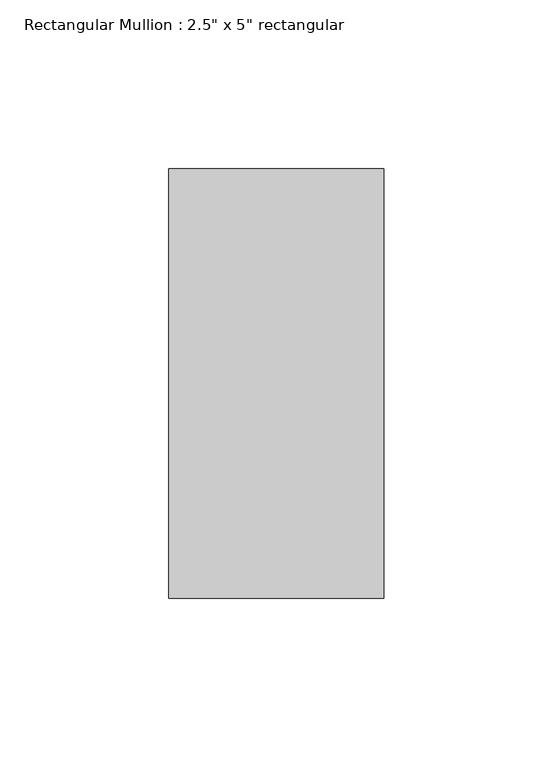
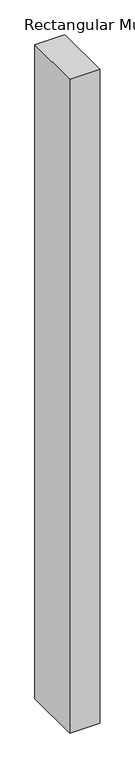
"""IFC4 building model written with IfcOpenShell, lengths in millimetres: member geometry."""

from ifc_helpers import new_model, si_unit, frame, origin, place, context, project, spatial, polyline, outline, extrude, source, transform, mapped, element, save


def member_a95d9ad3(model_context):
    return source(origin(), model_context, "Body", "SweptSolid", [
        extrude(outline(polyline([(31.75, 63.5), (31.75, -63.5), (-31.75, -63.5), (-31.75, 63.5), (31.75, 63.5)])), frame((0.0, 0.0, -1460.4999998), z_axis=(0.0, 0.0, 1.0), x_axis=(1.0, 0.0, 0.0)), (0.0, 0.0, 1.0), 1460.4999998),
    ])


if __name__ == "__main__":
    model = new_model("IFC4")
    model_context = context("Model", 3, world=origin())
    ifc_project = project(units=[si_unit("LENGTHUNIT", "METRE", prefix="MILLI")], contexts=[model_context])
    site = spatial("IfcSite", under=ifc_project)
    building = spatial("IfcBuilding", under=site)
    placement = place(None, origin())
    member_shape = member_a95d9ad3(model_context)
    element("IfcMember", 1, ObjectType="Rectangular Mullion : 2.5\" x 5\" rectangular", at=placement, inside=building, context=model_context, shape_type="MappedRepresentation", body=[
        mapped(member_shape, transform((0.0, 0.0, 0.0), x_axis=(1.0, 0.0, 0.0), y_axis=(0.0, 1.0, 0.0), z_axis=(0.0, 0.0, 1.0))),
    ])
    save(model, "model.ifc")

# Revit data of these elements
# Type "Rectangular Mullion : 2.5\" x 5\" rectangular"
#   built-in parameter 1007304 = 0.416667 (stored number, unit not read)
#   built-in parameter 1007301 = 0.104167 (stored number, unit not read)
#   built-in parameter 1007300 = 0.104167 (stored number, unit not read)
# Element 1 (IfcMember, "Rectangular Mullion : 2.5\" x 5\" rectangular")
#   Materials on its faces: "BLACK COLOUR"
# Materials
#   "BLACK COLOUR": class "Generic", colour RGB 120 120 120, transparency 0, Cost = 0
